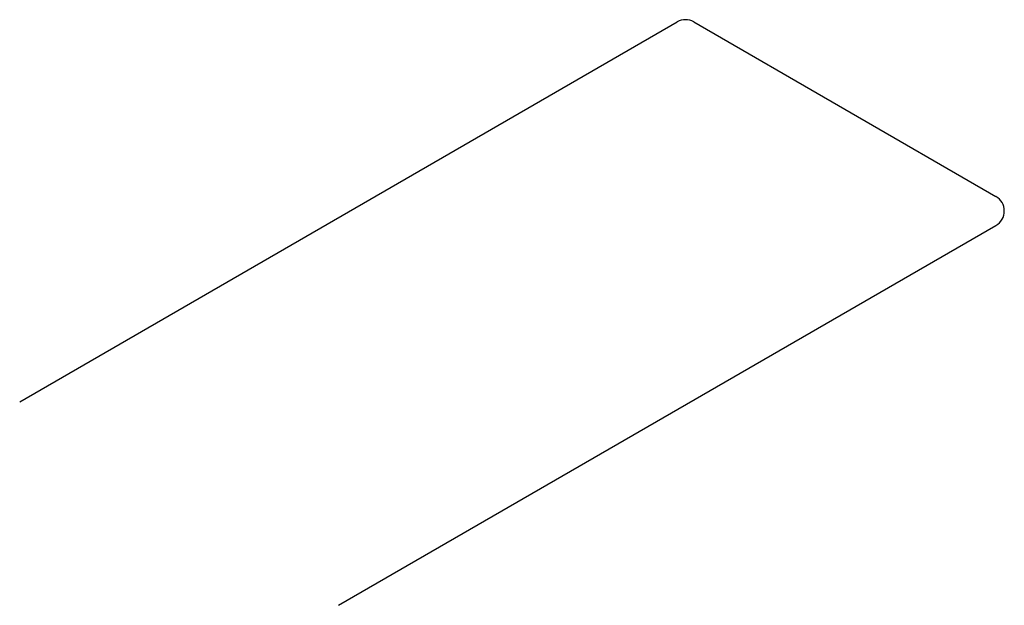
# Model space of a CAD drawing. Units: inches. Extents: x 5770 to 11891, y 3254 to 6808.
# Tile 15 of 15: x 11861 to 11891, y 6790 to 6808. Entities that reach past the tile are written whole.
import ezdxf

# ---------------------------------------------------------------- set-up
doc = ezdxf.new("R2010")
doc.units = ezdxf.units.IN
doc.layers.add('A-FURN', color=8, linetype='Continuous', lineweight=25)

msp = doc.modelspace()

# ---------------------------------------------------------------- linework, layer by layer
at = {"layer": 'A-FURN'}
for p, q in [((11861.199, 6796.057), (11880.984, 6807.479)), ((11881.484, 6807.479), (11890.577, 6802.229)), ((11870.793, 6789.94), (11890.577, 6801.363))]:
    msp.add_line(p, q, dxfattribs=at)
for centre, start, end in [((11881.234, 6807.046), 60, 120), ((11890.327, 6801.796), 300, 60)]:
    msp.add_arc(centre, 0.5, start, end, dxfattribs=at)

doc.saveas('drawing.dxf')
